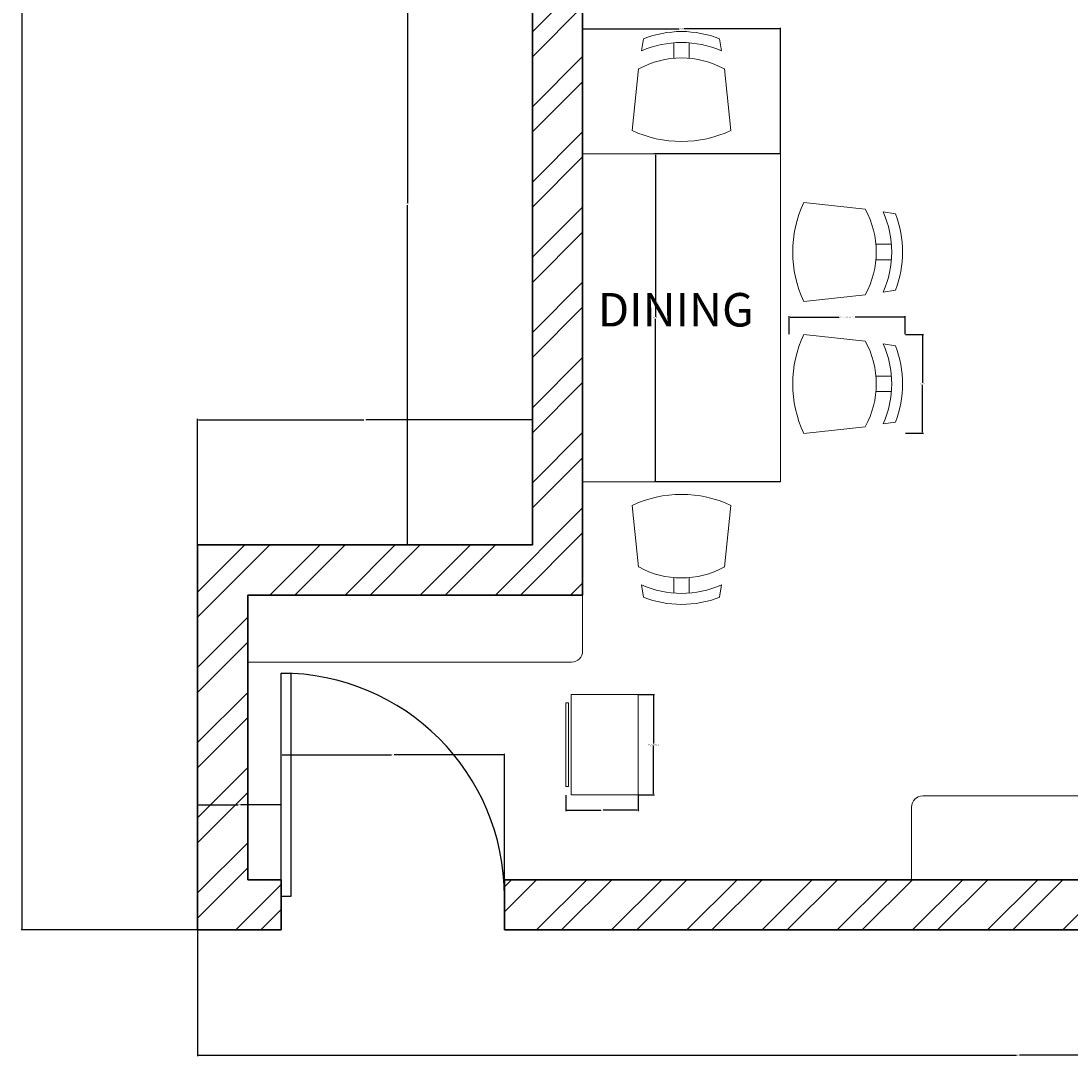
# Model space of a CAD drawing. Units: inches. Extents: x 3449 to 3843, y 1566 to 2054.
# Tile 1 of 8: x 3449 to 3638, y 1566 to 1751. Entities that reach past the tile are written whole.
import ezdxf

# ---------------------------------------------------------------- set-up
doc = ezdxf.new("R2010")
doc.units = ezdxf.units.IN
for name, color, linetype, lineweight in [('A-ANNO-DIMS', 2, 'Continuous', 18), ('A-AREA-IDEN', 7, 'Continuous', 25), ('A-DOOR', 4, 'Continuous', 25), ('A-FLOR-CASE', 7, 'Continuous', 20), ('A-WALL', 7, 'Continuous', 35), ('A-WALL-PATT', 251, 'Continuous', 13), ('furn', 7, 'Continuous', 18)]:
    doc.layers.add(name, color=color, linetype=linetype, lineweight=lineweight)
doc.styles.get("Standard").update_dxf_attribs({"font": 'arial.ttf'})
doc.dimstyles.get("Standard").update_dxf_attribs({"dimtxt": 0.18, "dimasz": 0.18, "dimexe": 0.18, "dimexo": 0.0625, "dimgap": 0.09, "dimtad": 0, "dimtih": 1, "dimtoh": 1, "dimdec": 4, "dimzin": 0, "dimdsep": 46, "dimtxsty": 'Standard', "dimcen": 0.09, "dimadec": 0, "dimazin": 0, "dimtfac": 1, "dimtdec": 4, "dimtofl": 0, "dimtmove": 0, "dimatfit": 3, "dimfxl": 1, "dimtolj": 1, "dimtzin": 0, "dimarcsym": 0})

# ---------------------------------------------------------------- blocks, each defined once
blk = doc.blocks.new('*U4')
for p, q in [((0, 0), (0, -6)), ((40, 0), (40, -6))]:
    blk.add_line(p, q)
blk.add_lwpolyline([(0, 0), (0, 40), (1.75, 40), (1.75, 0)], close=True)
blk.add_arc((0, 0), 40, 0, 90)
blk = doc.blocks.new('Wall Cabinet - 18 x 12 in side')
for points in [[(-12, -18), (-12, 0), (0, 0), (0, -18)], [(-13, -16.5), (-13, -1.5), (-12.5, -1.5), (-12.5, -16.5)]]:
    blk.add_lwpolyline(points, close=True)
blk = doc.blocks.new('CHAIR-DINING')
for p, q in [((0, 17.72), (1.18, 6.69)), ((17.72, 17.72), (16.54, 6.69)), ((7.48, 2.02), (7.48, 4.78)), ((10.24, 2.02), (10.24, 4.78)), ((1.68, 3.48), (2.03, 1.28)), ((16.03, 3.48), (15.69, 1.28))]:
    blk.add_line(p, q)
for centre, radius, start, end in [((8.86, -1.23), 20.92, 64.9424, 115.0576), ((8.86, 20.68), 15.95, 241.2372, 298.7628), ((8.86, 19.7), 17.74, 246.1344, 293.8656), ((8.86, 18.89), 18.89, 248.7887, 291.2113)]:
    blk.add_arc(centre, radius, start, end)
blk = doc.blocks.new('*D38')
at = {"layer": 'A-ANNO-DIMS', "color": 0, "lineweight": -2, "transparency": 16777216}
for p, q in [((3587.08, 1695.36), (3587.08, 1698.59)), ((3607.85, 1695.36), (3607.85, 1698.59)), ((3587.26, 1698.41), (3596.04, 1698.41)), ((3607.67, 1698.41), (3598.89, 1698.41))]:
    blk.add_line(p, q, dxfattribs=at)
at = {"layer": 'A-ANNO-DIMS', "color": 0, "transparency": 16777216}
for points in [[(3587.26, 1698.44), (3587.26, 1698.38), (3587.08, 1698.41)], [(3607.67, 1698.44), (3607.67, 1698.38), (3607.85, 1698.41)]]:
    blk.add_solid(points, dxfattribs=at)
at = {"layer": 'Defpoints', "color": 0, "transparency": 16777216}
for p in [(3587.08, 1698.41), (3587.08, 1695.29), (3607.85, 1695.29)]:
    blk.add_point(p, dxfattribs=at)
at = {"layer": 'A-ANNO-DIMS', "color": 0, "transparency": 16777216, "insert": (3597.46, 1698.41), "char_height": 0.18, "attachment_point": 5}
blk.add_mtext('\\A1;DINING CHAIR 21 TYP.', dxfattribs=at)
blk = doc.blocks.new('*D39')
at = {"layer": 'A-ANNO-DIMS', "color": 0, "lineweight": -2, "transparency": 16777216}
for p, q in [((3607.91, 1695.29), (3611.14, 1695.29)), ((3610.96, 1695.11), (3610.96, 1686.62)), ((3610.96, 1677.76), (3610.96, 1686.25)), ((3607.91, 1677.58), (3611.14, 1677.58))]:
    blk.add_line(p, q, dxfattribs=at)
at = {"layer": 'A-ANNO-DIMS', "color": 0, "transparency": 16777216}
for points in [[(3610.93, 1695.11), (3610.99, 1695.11), (3610.96, 1695.29)], [(3610.93, 1677.76), (3610.99, 1677.76), (3610.96, 1677.58)]]:
    blk.add_solid(points, dxfattribs=at)
at = {"layer": 'Defpoints', "color": 0, "transparency": 16777216}
for p in [(3607.85, 1695.29), (3610.96, 1695.29), (3607.85, 1677.58)]:
    blk.add_point(p, dxfattribs=at)
at = {"layer": 'A-ANNO-DIMS', "color": 0, "transparency": 16777216, "insert": (3610.96, 1686.44), "char_height": 0.18, "attachment_point": 5}
blk.add_mtext('\\A1;18 TYP.', dxfattribs=at)
blk = doc.blocks.new('*D72')
at = {"layer": 'A-ANNO-DIMS', "color": 0, "lineweight": -2, "transparency": 16777216}
for p, q in [((3560.13, 1630.8), (3562.95, 1630.8)), ((3562.77, 1630.62), (3562.77, 1621.99)), ((3562.77, 1612.98), (3562.77, 1621.62)), ((3560.13, 1612.8), (3562.95, 1612.8))]:
    blk.add_line(p, q, dxfattribs=at)
at = {"layer": 'A-ANNO-DIMS', "color": 0, "transparency": 16777216}
for points in [[(3562.74, 1630.62), (3562.8, 1630.62), (3562.77, 1630.8)], [(3562.74, 1612.98), (3562.8, 1612.98), (3562.77, 1612.8)]]:
    blk.add_solid(points, dxfattribs=at)
at = {"layer": 'Defpoints', "color": 0, "transparency": 16777216}
for p in [(3560.07, 1630.8), (3562.77, 1630.8), (3560.07, 1612.8)]:
    blk.add_point(p, dxfattribs=at)
at = {"layer": 'A-ANNO-DIMS', "color": 0, "transparency": 16777216, "insert": (3562.77, 1621.8), "char_height": 0.18, "attachment_point": 5}
blk.add_mtext('\\A1;WALL CABINET 18', dxfattribs=at)
blk = doc.blocks.new('*D73')
at = {"layer": 'A-ANNO-DIMS', "color": 0, "lineweight": -2, "transparency": 16777216}
for p, q in [((3547.07, 1612.74), (3547.07, 1609.92)), ((3560.07, 1612.74), (3560.07, 1609.92)), ((3547.25, 1610.1), (3553.36, 1610.1)), ((3559.89, 1610.1), (3553.78, 1610.1))]:
    blk.add_line(p, q, dxfattribs=at)
at = {"layer": 'A-ANNO-DIMS', "color": 0, "transparency": 16777216}
for points in [[(3547.25, 1610.13), (3547.25, 1610.07), (3547.07, 1610.1)], [(3559.89, 1610.13), (3559.89, 1610.07), (3560.07, 1610.1)]]:
    blk.add_solid(points, dxfattribs=at)
at = {"layer": 'Defpoints', "color": 0, "transparency": 16777216}
for p in [(3547.07, 1612.8), (3560.07, 1612.8), (3560.07, 1610.1)]:
    blk.add_point(p, dxfattribs=at)
at = {"layer": 'A-ANNO-DIMS', "color": 0, "transparency": 16777216, "insert": (3553.57, 1610.1), "char_height": 0.18, "attachment_point": 5}
blk.add_mtext('\\A1;13', dxfattribs=at)
blk = doc.blocks.new('*D77')
at = {"layer": 'A-ANNO-DIMS', "color": 0, "lineweight": -2, "transparency": 16777216}
for p, q in [((3472.03, 2031.61), (3449.51, 2031.61)), ((3449.69, 2031.43), (3449.69, 1810.3)), ((3449.69, 1588.79), (3449.69, 1809.93)), ((3481.03, 1588.61), (3449.51, 1588.61))]:
    blk.add_line(p, q, dxfattribs=at)
at = {"layer": 'A-ANNO-DIMS', "color": 0, "transparency": 16777216}
for points in [[(3449.66, 2031.43), (3449.72, 2031.43), (3449.69, 2031.61)], [(3449.66, 1588.79), (3449.72, 1588.79), (3449.69, 1588.61)]]:
    blk.add_solid(points, dxfattribs=at)
at = {"layer": 'Defpoints', "color": 0, "transparency": 16777216}
for p in [(3449.69, 2031.61), (3472.09, 2031.61), (3481.09, 1588.61)]:
    blk.add_point(p, dxfattribs=at)
at = {"layer": 'A-ANNO-DIMS', "color": 0, "transparency": 16777216, "insert": (3449.69, 1810.11), "char_height": 0.18, "attachment_point": 5}
blk.add_mtext('\\A1;443', dxfattribs=at)
blk = doc.blocks.new('*D96')
at = {"layer": 'A-ANNO-DIMS', "color": 0, "lineweight": -2, "transparency": 16777216}
for p, q in [((3541.03, 1779.61), (3518.51, 1779.61)), ((3518.69, 1779.43), (3518.69, 1718.79)), ((3518.69, 1657.79), (3518.69, 1718.43)), ((3541.03, 1657.61), (3518.51, 1657.61))]:
    blk.add_line(p, q, dxfattribs=at)
at = {"layer": 'A-ANNO-DIMS', "color": 0, "transparency": 16777216}
for points in [[(3518.66, 1779.43), (3518.72, 1779.43), (3518.69, 1779.61)], [(3518.66, 1657.79), (3518.72, 1657.79), (3518.69, 1657.61)]]:
    blk.add_solid(points, dxfattribs=at)
at = {"layer": 'Defpoints', "color": 0, "transparency": 16777216}
for p in [(3518.69, 1779.61), (3541.09, 1779.61), (3541.09, 1657.61)]:
    blk.add_point(p, dxfattribs=at)
at = {"layer": 'A-ANNO-DIMS', "color": 0, "transparency": 16777216, "insert": (3518.69, 1718.61), "char_height": 0.18, "attachment_point": 5}
blk.add_mtext('\\A1;122', dxfattribs=at)
blk = doc.blocks.new('*D97')
at = {"layer": 'A-ANNO-DIMS', "color": 0, "lineweight": -2, "transparency": 16777216}
for p, q in [((3481.09, 1657.68), (3481.09, 1680.19)), ((3481.27, 1680.01), (3510.87, 1680.01)), ((3540.91, 1680.01), (3511.31, 1680.01)), ((3541.09, 1657.68), (3541.09, 1680.19))]:
    blk.add_line(p, q, dxfattribs=at)
at = {"layer": 'A-ANNO-DIMS', "color": 0, "transparency": 16777216}
for points in [[(3481.27, 1680.04), (3481.27, 1679.98), (3481.09, 1680.01)], [(3540.91, 1680.04), (3540.91, 1679.98), (3541.09, 1680.01)]]:
    blk.add_solid(points, dxfattribs=at)
at = {"layer": 'Defpoints', "color": 0, "transparency": 16777216}
for p in [(3541.09, 1680.01), (3481.09, 1657.61), (3541.09, 1657.61)]:
    blk.add_point(p, dxfattribs=at)
at = {"layer": 'A-ANNO-DIMS', "color": 0, "transparency": 16777216, "insert": (3511.09, 1680.01), "char_height": 0.18, "attachment_point": 5}
blk.add_mtext('\\A1;60', dxfattribs=at)
blk = doc.blocks.new('*D98')
at = {"layer": 'A-ANNO-DIMS', "color": 0, "lineweight": -2, "transparency": 16777216}
for p, q in [((3496.09, 1597.68), (3496.09, 1620.19)), ((3496.27, 1620.01), (3515.87, 1620.01)), ((3535.91, 1620.01), (3516.31, 1620.01)), ((3536.09, 1597.68), (3536.09, 1620.19))]:
    blk.add_line(p, q, dxfattribs=at)
at = {"layer": 'A-ANNO-DIMS', "color": 0, "transparency": 16777216}
for points in [[(3496.27, 1620.04), (3496.27, 1619.98), (3496.09, 1620.01)], [(3535.91, 1620.04), (3535.91, 1619.98), (3536.09, 1620.01)]]:
    blk.add_solid(points, dxfattribs=at)
at = {"layer": 'Defpoints', "color": 0, "transparency": 16777216}
for p in [(3536.09, 1620.01), (3496.09, 1597.61), (3536.09, 1597.61)]:
    blk.add_point(p, dxfattribs=at)
at = {"layer": 'A-ANNO-DIMS', "color": 0, "transparency": 16777216, "insert": (3516.09, 1620.01), "char_height": 0.18, "attachment_point": 5}
blk.add_mtext('\\A1;40', dxfattribs=at)
blk = doc.blocks.new('*D99')
at = {"layer": 'A-ANNO-DIMS', "color": 0, "lineweight": -2, "transparency": 16777216}
for p, q in [((3481.09, 1588.55), (3481.09, 1566.03)), ((3775.09, 1588.55), (3775.09, 1566.03)), ((3481.27, 1566.21), (3627.8, 1566.21)), ((3774.91, 1566.21), (3628.38, 1566.21))]:
    blk.add_line(p, q, dxfattribs=at)
at = {"layer": 'A-ANNO-DIMS', "color": 0, "transparency": 16777216}
for points in [[(3481.27, 1566.24), (3481.27, 1566.18), (3481.09, 1566.21)], [(3774.91, 1566.24), (3774.91, 1566.18), (3775.09, 1566.21)]]:
    blk.add_solid(points, dxfattribs=at)
at = {"layer": 'Defpoints', "color": 0, "transparency": 16777216}
for p in [(3481.09, 1588.61), (3775.09, 1588.61), (3481.09, 1566.21)]:
    blk.add_point(p, dxfattribs=at)
at = {"layer": 'A-ANNO-DIMS', "color": 0, "transparency": 16777216, "insert": (3628.09, 1566.21), "char_height": 0.18, "attachment_point": 5}
blk.add_mtext('\\A1;294', dxfattribs=at)
blk = doc.blocks.new('*D107')
at = {"layer": 'A-ANNO-DIMS', "color": 0, "lineweight": -2, "transparency": 16777216}
for p, q in [((3550.09, 1727.68), (3550.09, 1750.2)), ((3550.27, 1750.02), (3567.41, 1750.02)), ((3585.34, 1750.02), (3568.2, 1750.02)), ((3585.52, 1727.68), (3585.52, 1750.2))]:
    blk.add_line(p, q, dxfattribs=at)
at = {"layer": 'A-ANNO-DIMS', "color": 0, "transparency": 16777216}
for points in [[(3550.27, 1750.05), (3550.27, 1749.99), (3550.09, 1750.02)], [(3585.34, 1750.05), (3585.34, 1749.99), (3585.52, 1750.02)]]:
    blk.add_solid(points, dxfattribs=at)
at = {"layer": 'Defpoints', "color": 0, "transparency": 16777216}
for p in [(3585.52, 1750.02), (3550.09, 1727.62), (3585.52, 1727.62)]:
    blk.add_point(p, dxfattribs=at)
at = {"layer": 'A-ANNO-DIMS', "color": 0, "transparency": 16777216, "insert": (3567.8, 1750.02), "char_height": 0.18, "attachment_point": 5}
blk.add_mtext('\\A1;35.43', dxfattribs=at)
blk = doc.blocks.new('*D108')
at = {"layer": 'A-ANNO-DIMS', "color": 0, "lineweight": -2, "transparency": 16777216}
for p, q in [((3585.46, 1727.62), (3562.94, 1727.62)), ((3563.12, 1727.44), (3563.12, 1698.43)), ((3563.12, 1669.05), (3563.12, 1698.06)), ((3585.46, 1668.87), (3562.94, 1668.87))]:
    blk.add_line(p, q, dxfattribs=at)
at = {"layer": 'A-ANNO-DIMS', "color": 0, "transparency": 16777216}
for points in [[(3563.09, 1727.44), (3563.15, 1727.44), (3563.12, 1727.62)], [(3563.09, 1669.05), (3563.15, 1669.05), (3563.12, 1668.87)]]:
    blk.add_solid(points, dxfattribs=at)
at = {"layer": 'Defpoints', "color": 0, "transparency": 16777216}
for p in [(3563.12, 1727.62), (3585.52, 1727.62), (3585.52, 1668.87)]:
    blk.add_point(p, dxfattribs=at)
at = {"layer": 'A-ANNO-DIMS', "color": 0, "transparency": 16777216, "insert": (3563.12, 1698.25), "char_height": 0.18, "attachment_point": 5}
blk.add_mtext('\\A1;58.75', dxfattribs=at)
blk = doc.blocks.new('*D114')
at = {"layer": 'A-ANNO-DIMS', "color": 0, "lineweight": -2, "transparency": 16777216}
for p, q in [((3481.09, 1588.68), (3481.09, 1611.19)), ((3481.27, 1611.01), (3488.38, 1611.01)), ((3495.91, 1611.01), (3488.8, 1611.01)), ((3496.09, 1588.68), (3496.09, 1611.19))]:
    blk.add_line(p, q, dxfattribs=at)
at = {"layer": 'A-ANNO-DIMS', "color": 0, "transparency": 16777216}
for points in [[(3481.27, 1611.04), (3481.27, 1610.98), (3481.09, 1611.01)], [(3495.91, 1611.04), (3495.91, 1610.98), (3496.09, 1611.01)]]:
    blk.add_solid(points, dxfattribs=at)
at = {"layer": 'Defpoints', "color": 0, "transparency": 16777216}
for p in [(3496.09, 1611.01), (3481.09, 1588.61), (3496.09, 1588.61)]:
    blk.add_point(p, dxfattribs=at)
at = {"layer": 'A-ANNO-DIMS', "color": 0, "transparency": 16777216, "insert": (3488.59, 1611.01), "char_height": 0.18, "attachment_point": 5}
blk.add_mtext('\\A1;15', dxfattribs=at)

msp = doc.modelspace()

# ---------------------------------------------------------------- hatches: boundary and pattern name
at = {"layer": 'A-WALL-PATT'}
h = msp.add_hatch(dxfattribs=at)
h.set_pattern_fill('ANSI32', color=256)
edge = h.paths.add_edge_path()
edge.add_line((3481.088, 2022.6144), (3508.088, 2022.6144))
edge.add_line((3508.088, 2022.6144), (3508.088, 2031.6144))
edge.add_line((3508.088, 2031.6144), (3472.088, 2031.6144))
edge.add_line((3472.088, 2031.6144), (3472.088, 1779.6144))
edge.add_line((3472.088, 1779.6144), (3481.088, 1779.6144))
edge.add_line((3481.088, 1779.6144), (3481.088, 1839.6144))
edge.add_line((3481.088, 1839.6144), (3571.088, 1839.6144))
edge.add_line((3571.088, 1839.6144), (3571.088, 1824.3194))
edge.add_line((3571.088, 1824.3194), (3571.088, 1821.6144))
edge.add_line((3571.088, 1821.6144), (3580.088, 1821.6144))
edge.add_line((3580.088, 1821.6144), (3580.088, 1825.1908))
edge.add_ellipse((3580.1411, 1825.2442), major_axis=(0, 0.0754), ratio=0.99913951, start_angle=90, end_angle=135.183195, ccw=False)
edge.add_line((3580.0017, 1825.3196), (3580.0658, 1825.3196))
edge.add_line((3580.0658, 1825.3196), (3580.066, 1839.6365))
edge.add_line((3580.066, 1839.6365), (3616.088, 1839.6365))
edge.add_line((3616.088, 1839.6365), (3616.088, 1848.6144))
edge.add_line((3616.088, 1848.6144), (3610.088, 1848.6144))
edge.add_line((3610.088, 1848.6144), (3574.088, 1848.6144))
edge.add_line((3574.088, 1848.6144), (3481.088, 1848.6144))
edge.add_line((3481.088, 1848.6144), (3481.088, 1872.6144))
edge.add_line((3481.088, 1872.6144), (3481.088, 2022.6144))
h.paths.add_polyline_path([(3550.088, 1779.6144), (3616.088, 1779.6144), (3616.088, 1791.6144), (3505.088, 1791.6144), (3505.088, 1779.6144), (3541.088, 1779.6144), (3541.088, 1657.6144), (3481.088, 1657.6144), (3481.088, 1588.6144), (3496.088, 1588.6144), (3496.088, 1594.6144), (3496.088, 1597.6144), (3490.088, 1597.6144), (3490.088, 1648.6144), (3550.088, 1648.6144)])
h.paths.add_polyline_path([(3775.088, 1612.6144), (3766.088, 1612.6144), (3766.088, 1597.6144), (3536.088, 1597.6144), (3536.088, 1588.6144), (3775.088, 1588.6144)])
h.paths.add_polyline_path([(3820.088, 1756.6144), (3811.088, 1756.6144), (3811.088, 1732.6144), (3664.088, 1732.6144), (3664.088, 1723.6144), (3766.088, 1723.6144), (3766.088, 1708.6144), (3775.088, 1708.6144), (3775.088, 1723.6144), (3820.088, 1723.6144)])
h.paths.add_polyline_path([(3820.088, 1986.6144), (3745.088, 1986.6144), (3745.088, 2010.6144), (3664.088, 2010.6144), (3664.088, 1992.6144), (3652.088, 1992.6144), (3652.088, 1983.6144), (3664.088, 1983.6144), (3664.088, 1893.6144), (3648.793, 1893.6144), (3607.088, 1893.6144), (3607.088, 1884.6144), (3673.088, 1884.6144), (3673.088, 2001.6144), (3736.088, 2001.6144), (3736.088, 1977.6144), (3811.088, 1977.6144), (3811.088, 1949.1144), (3820.088, 1949.1144)])
h.paths.add_polyline_path([(3628.088, 1992.6144), (3616.088, 1992.6144), (3616.088, 2031.6144), (3580.088, 2031.6144), (3580.088, 2022.6144), (3607.088, 2022.6144), (3607.088, 1921.6144), (3613.088, 1921.6144), (3616.088, 1921.6144), (3616.088, 1983.6144), (3628.088, 1983.6144)])
h.paths.add_polyline_path([(3820.088, 1877.1144), (3811.088, 1877.1144), (3811.088, 1848.6144), (3664.088, 1848.6144), (3664.088, 1839.6144), (3700.088, 1839.6144), (3811.088, 1839.6144), (3811.088, 1815.6144), (3820.088, 1815.6144)])

# ---------------------------------------------------------------- linework, layer by layer
at = {"layer": 'A-FLOR-CASE'}
for p, q in [((3550.088, 1648.6144), (3550.088, 1638.6144)), ((3490.088, 1636.6144), (3548.088, 1636.6144))]:
    msp.add_line(p, q, dxfattribs=at)
msp.add_arc((3548.088, 1638.6144), 2, 270, 0, dxfattribs=at)
at = {"layer": 'A-WALL'}
for p, q in [((3541.088, 1779.6144), (3541.088, 1657.6144)), ((3550.088, 1779.6144), (3550.088, 1648.6144)), ((3481.088, 1657.6144), (3481.088, 1588.6144)), ((3481.088, 1657.6144), (3541.088, 1657.6144)), ((3490.088, 1648.6144), (3490.088, 1597.6144)), ((3490.088, 1648.6144), (3550.088, 1648.6144)), ((3490.088, 1597.6144), (3496.088, 1597.6144)), ((3496.088, 1597.6144), (3496.088, 1588.6144)), ((3536.088, 1597.6144), (3536.088, 1588.6144)), ((3536.088, 1597.6144), (3766.088, 1597.6144)), ((3481.088, 1588.6144), (3496.088, 1588.6144)), ((3536.088, 1588.6144), (3775.088, 1588.6144))]:
    msp.add_line(p, q, dxfattribs=at)
at = {"layer": 'furn'}
for p, q in [((3550.088, 1668.8701), (3550.088, 1727.622)), ((3550.088, 1727.622), (3585.5211, 1727.622)), ((3585.5211, 1668.8701), (3585.5211, 1727.622)), ((3550.088, 1668.8701), (3585.5211, 1668.8701))]:
    msp.add_line(p, q, dxfattribs=at)
msp.add_lwpolyline([(3609.0062, 1597.6144), (3642.0062, 1597.6144), (3642.0062, 1610.6144, 0.41421356), (3640.0062, 1612.6144), (3611.0062, 1612.6144, 0.41421356), (3609.0062, 1610.6144)], format="xyb", close=True, dxfattribs=at)

# ---------------------------------------------------------------- block references
at = {"layer": 'A-DOOR'}
msp.add_blockref('*U4', (3496.088, 1594.6144), dxfattribs=at)
at = {"layer": 'A-FLOR-CASE'}
msp.add_blockref('Wall Cabinet - 18 x 12 in side', (3560.0658, 1630.8035), dxfattribs=at)
at = {"layer": 'furn'}
for p, rotation in [((3576.6631, 1749.5521), 180), ((3607.4199, 1701.1985), 89.99999999999883), ((3607.4199, 1677.5765), 90.00000000000291)]:
    msp.add_blockref('CHAIR-DINING', p, dxfattribs=dict(at, rotation=rotation))
msp.add_blockref('CHAIR-DINING', (3558.946, 1646.94), dxfattribs=at)

# ---------------------------------------------------------------- texts
at = {"layer": 'A-AREA-IDEN', "insert": (3552.8048, 1702.7163), "char_height": 6, "attachment_point": 1}
msp.add_mtext_dynamic_manual_height_columns('DINING', width=95.638287, gutter_width=12.5, heights=[0], dxfattribs=at)

# ---------------------------------------------------------------- dimensions: what is measured, and where the dimension line sits
at = {"layer": 'A-ANNO-DIMS'}
for base, p1, p2, angle, override, picture, middle in [((3449.688, 2031.6144), (3481.088, 1588.6144), (3472.088, 2031.6144), 90, {"dimdec": 0, "dimlfac": 1, "dimrnd": 0, "dimzin": 0, "dimdsep": 46, "dimlunit": 2}, '*D77', (3449.688, 1810.1144)), ((3518.688, 1779.6144), (3541.088, 1657.6144), (3541.088, 1779.6144), 90, {"dimdec": 0, "dimlfac": 1, "dimrnd": 0, "dimzin": 0, "dimdsep": 46, "dimlunit": 2}, '*D96', (3518.688, 1718.6144)), ((3563.1211, 1727.622), (3585.5211, 1668.8701), (3585.5211, 1727.622), 90, {"dimdec": 2, "dimlfac": 1, "dimrnd": 0, "dimzin": 0, "dimdsep": 46, "dimlunit": 2}, '*D108', (3563.1211, 1698.246)), ((3481.088, 1566.2144), (3775.088, 1588.6144), (3481.088, 1588.6144), 180, {"dimdec": 0, "dimlfac": 1, "dimrnd": 0, "dimzin": 0, "dimdsep": 46, "dimlunit": 2}, '*D99', (3628.088, 1566.2144))]:
    dim = msp.add_linear_dim(base=base, p1=p1, p2=p2, angle=angle, dimstyle='Standard', override=override, dxfattribs=at)
    dim.commit()
    dim.dimension.update_dxf_attribs({"geometry": picture, "text_midpoint": middle})
for base, p1, p2, override, picture, middle in [((3585.5211, 1750.022), (3550.088, 1727.622), (3585.5211, 1727.622), {"dimdec": 2, "dimlfac": 1, "dimrnd": 0, "dimzin": 0, "dimdsep": 46, "dimlunit": 2}, '*D107', (3567.8046, 1750.022)), ((3541.088, 1680.0144), (3481.088, 1657.6144), (3541.088, 1657.6144), {"dimdec": 0, "dimlfac": 1, "dimrnd": 0, "dimzin": 0, "dimdsep": 46, "dimlunit": 2}, '*D97', (3511.088, 1680.0144)), ((3536.088, 1620.0144), (3496.088, 1597.6144), (3536.088, 1597.6144), {"dimdec": 0, "dimlfac": 1, "dimrnd": 0, "dimzin": 0, "dimdsep": 46, "dimlunit": 2}, '*D98', (3516.088, 1620.0144)), ((3560.0658, 1610.1035), (3547.0658, 1612.8035), (3560.0658, 1612.8035), {"dimdec": 0, "dimlfac": 1, "dimrnd": 0, "dimzin": 0, "dimdsep": 46, "dimlunit": 2}, '*D73', (3553.5658, 1610.1035)), ((3496.088, 1611.0144), (3481.088, 1588.6144), (3496.088, 1588.6144), {"dimdec": 0, "dimlfac": 1, "dimrnd": 0, "dimzin": 0, "dimdsep": 46, "dimlunit": 2}, '*D114', (3488.588, 1611.0144))]:
    dim = msp.add_linear_dim(base=base, p1=p1, p2=p2, dimstyle='Standard', override=override, dxfattribs=at)
    dim.commit()
    dim.dimension.update_dxf_attribs({"geometry": picture, "text_midpoint": middle})
for base, p1, p2, angle, text, picture, middle in [((3587.079, 1698.4085), (3607.8468, 1695.2933), (3587.079, 1695.2933), 180, 'DINING CHAIR <> TYP.', '*D38', (3597.4629, 1698.4085)), ((3610.9619, 1695.2933), (3607.8468, 1677.5767), (3607.8468, 1695.2933), 90, '<> TYP.', '*D39', (3610.9619, 1686.435)), ((3562.7658, 1630.8035), (3560.0658, 1612.8035), (3560.0658, 1630.8035), 90, 'WALL CABINET <>', '*D72', (3562.7658, 1621.8035))]:
    dim = msp.add_linear_dim(base=base, p1=p1, p2=p2, angle=angle, text=text, dimstyle='Standard', override={"dimdec": 0, "dimlfac": 1, "dimrnd": 0, "dimzin": 0, "dimdsep": 46, "dimlunit": 2}, dxfattribs=at)
    dim.commit()
    dim.dimension.update_dxf_attribs({"geometry": picture, "text_midpoint": middle})

doc.saveas('drawing.dxf')
